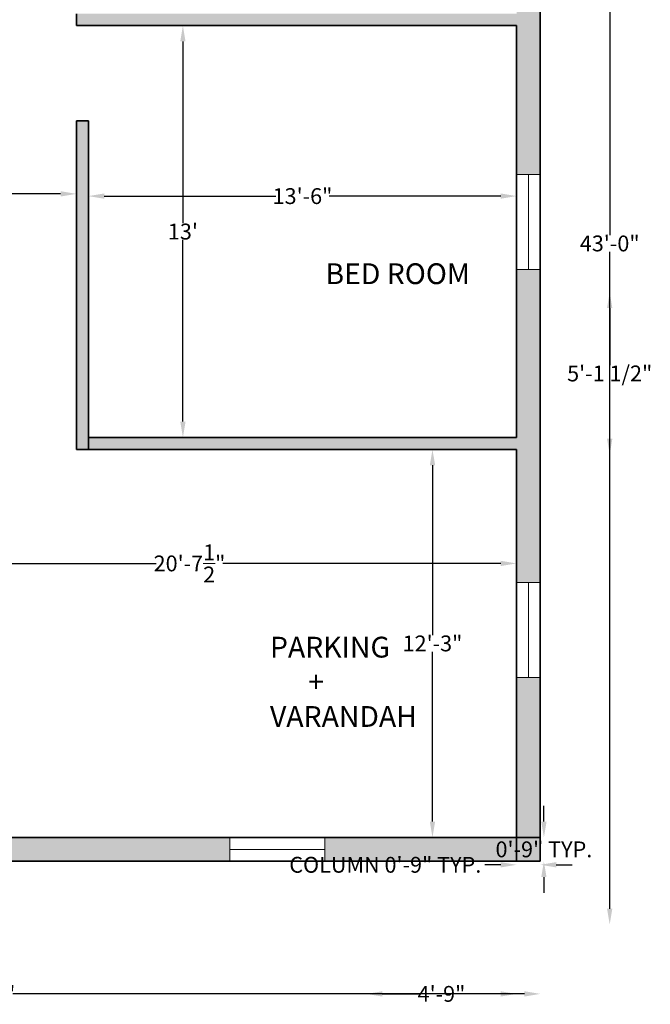
# Model space of a CAD drawing. Units: inches. Extents: x 759 to 1283, y 452 to 1038.
# Tile 2 of 3: x 1044 to 1283, y 457 to 830. Entities that reach past the tile are written whole.
import ezdxf

# ---------------------------------------------------------------- set-up
doc = ezdxf.new("R2010")
doc.units = ezdxf.units.IN
for name, color, linetype, lineweight in [('A-AREA-IDEN', 1, 'Continuous', 25), ('A-COLS', 7, 'Continuous', 35), ('A-COLS-PATT', 7, 'Continuous', 13), ('DIM', 2, 'Continuous', 18), ('WALL', 7, 'Continuous', 35), ('WINDOWS', 4, 'Continuous', 18)]:
    doc.layers.add(name, color=color, linetype=linetype, lineweight=lineweight)
doc.layers.add('A-WALL-PATT', color=67, linetype='Continuous', lineweight=13, true_color=0x727430)
doc.styles.get("Standard").update_dxf_attribs({"font": 'arial.ttf'})
doc.dimstyles.get("Standard").update_dxf_attribs({"dimtxt": 6, "dimasz": 6, "dimexe": 0.18, "dimexo": 0.0625, "dimgap": 0.09, "dimtad": 0, "dimtih": 1, "dimtoh": 1, "dimdec": 4, "dimzin": 0, "dimdsep": 46, "dimlunit": 4, "dimtxsty": 'Standard', "dimcen": 0.09, "dimse1": 1, "dimse2": 1, "dimadec": 0, "dimazin": 0, "dimtfac": 1, "dimtdec": 4, "dimtofl": 0, "dimtmove": 0, "dimatfit": 3, "dimfxl": 1, "dimtolj": 1, "dimtzin": 0, "dimarcsym": 0})

# ---------------------------------------------------------------- blocks, each defined once
blk = doc.blocks.new('*D11')
at = {"layer": 'Defpoints', "color": 0, "transparency": 16777216}
for p in [(1232.47, 666.81), (1200.66, 519.81), (1232.47, 519.81)]:
    blk.add_point(p, dxfattribs=at)
at = {"layer": 'DIM', "color": 0, "lineweight": -2, "transparency": 16777216}
for p, q in [((1200.66, 660.81), (1200.66, 596.46)), ((1200.66, 525.81), (1200.66, 590.15))]:
    blk.add_line(p, q, dxfattribs=at)
at = {"layer": 'DIM', "color": 0, "transparency": 16777216}
for points in [[(1199.66, 660.81), (1201.66, 660.81), (1200.66, 666.81)], [(1199.66, 525.81), (1201.66, 525.81), (1200.66, 519.81)]]:
    blk.add_solid(points, dxfattribs=at)
at = {"layer": 'DIM', "color": 0, "transparency": 16777216, "insert": (1200.66, 593.31), "char_height": 6, "attachment_point": 5}
blk.add_mtext('\\A1;12\'-3"', dxfattribs=at)
blk = doc.blocks.new('*D12')
at = {"layer": 'Defpoints', "color": 0, "transparency": 16777216}
for p in [(1232.47, 623.61), (984.97, 524.08), (1232.47, 524.08)]:
    blk.add_point(p, dxfattribs=at)
at = {"layer": 'DIM', "color": 0, "lineweight": -2, "transparency": 16777216}
for p, q in [((990.97, 623.61), (1096.08, 623.61)), ((1226.47, 623.61), (1121.35, 623.61))]:
    blk.add_line(p, q, dxfattribs=at)
at = {"layer": 'DIM', "color": 0, "transparency": 16777216}
for points in [[(990.97, 624.61), (990.97, 622.61), (984.97, 623.61)], [(1226.47, 624.61), (1226.47, 622.61), (1232.47, 623.61)]]:
    blk.add_solid(points, dxfattribs=at)
at = {"layer": 'DIM', "color": 0, "transparency": 16777216, "insert": (1108.72, 623.61), "char_height": 6, "attachment_point": 5}
blk.add_mtext('\\A1;20\'-7{\\H1x;\\S1/2;}"', dxfattribs=at)
blk = doc.blocks.new('*D13')
at = {"layer": 'Defpoints', "color": 0, "transparency": 16777216}
for p in [(1106.22, 827.31), (1215.11, 827.31), (1215.11, 671.31)]:
    blk.add_point(p, dxfattribs=at)
at = {"layer": 'DIM', "color": 0, "lineweight": -2, "transparency": 16777216}
for p, q in [((1106.22, 821.31), (1106.22, 752.46)), ((1106.22, 677.31), (1106.22, 746.15))]:
    blk.add_line(p, q, dxfattribs=at)
at = {"layer": 'DIM', "color": 0, "transparency": 16777216}
for points in [[(1105.22, 821.31), (1107.22, 821.31), (1106.22, 827.31)], [(1105.22, 677.31), (1107.22, 677.31), (1106.22, 671.31)]]:
    blk.add_solid(points, dxfattribs=at)
at = {"layer": 'DIM', "color": 0, "transparency": 16777216, "insert": (1106.22, 749.31), "char_height": 6, "attachment_point": 5}
blk.add_mtext("\\A1;13'", dxfattribs=at)
blk = doc.blocks.new('*D14')
at = {"layer": 'Defpoints', "color": 0, "transparency": 16777216}
for p in [(1070.47, 775.52), (1232.47, 775.52), (1232.47, 762.74)]:
    blk.add_point(p, dxfattribs=at)
at = {"layer": 'DIM', "color": 0, "lineweight": -2, "transparency": 16777216}
for p, q in [((1076.47, 762.74), (1141.35, 762.74)), ((1226.47, 762.74), (1161.58, 762.74))]:
    blk.add_line(p, q, dxfattribs=at)
at = {"layer": 'DIM', "color": 0, "transparency": 16777216}
for points in [[(1076.47, 763.74), (1076.47, 761.74), (1070.47, 762.74)], [(1226.47, 763.74), (1226.47, 761.74), (1232.47, 762.74)]]:
    blk.add_solid(points, dxfattribs=at)
at = {"layer": 'DIM', "color": 0, "transparency": 16777216, "insert": (1151.47, 762.74), "char_height": 6, "attachment_point": 5}
blk.add_mtext('\\A1;13\'-6"', dxfattribs=at)
blk = doc.blocks.new('*D15')
at = {"layer": 'Defpoints', "color": 0, "transparency": 16777216}
for p in [(1065.97, 763.58), (918.97, 756.35), (1065.97, 756.35)]:
    blk.add_point(p, dxfattribs=at)
at = {"layer": 'DIM', "color": 0, "lineweight": -2, "transparency": 16777216}
for p, q in [((924.97, 763.58), (982.35, 763.58)), ((1059.97, 763.58), (1002.58, 763.58))]:
    blk.add_line(p, q, dxfattribs=at)
at = {"layer": 'DIM', "color": 0, "transparency": 16777216}
for points in [[(924.97, 764.58), (924.97, 762.58), (918.97, 763.58)], [(1059.97, 764.58), (1059.97, 762.58), (1065.97, 763.58)]]:
    blk.add_solid(points, dxfattribs=at)
at = {"layer": 'DIM', "color": 0, "transparency": 16777216, "insert": (992.47, 763.58), "char_height": 6, "attachment_point": 5}
blk.add_mtext('\\A1;12\'-3"', dxfattribs=at)
blk = doc.blocks.new('WIN-36IN')
for p, q in [((0, 0), (0, 9)), ((0, 9), (36, 9)), ((36, 9), (36, 0)), ((0, 4.5), (36, 4.5)), ((36, 0), (0, 0))]:
    blk.add_line(p, q)
blk = doc.blocks.new('COL-9X9IN')
for p, q in [((0, 0), (0, 9)), ((0, 9), (9, 9)), ((9, 9), (9, 0)), ((9, 0), (0, 0))]:
    blk.add_line(p, q)
blk = doc.blocks.new('*D21')
at = {"layer": 'Defpoints', "color": 0, "transparency": 16777216}
for p in [(1232.47, 510.81), (1232.47, 509.46), (1241.47, 510.81)]:
    blk.add_point(p, dxfattribs=at)
at = {"layer": 'DIM', "color": 0, "lineweight": -2, "transparency": 16777216}
for p, q in [((1226.47, 509.46), (1220.47, 509.46)), ((1247.47, 509.46), (1253.47, 509.46))]:
    blk.add_line(p, q, dxfattribs=at)
at = {"layer": 'DIM', "color": 0, "transparency": 16777216}
for points in [[(1226.47, 510.46), (1226.47, 508.46), (1232.47, 509.46)], [(1247.47, 510.46), (1247.47, 508.46), (1241.47, 509.46)]]:
    blk.add_solid(points, dxfattribs=at)
at = {"layer": 'DIM', "color": 0, "transparency": 16777216, "insert": (1182.8, 509.46), "char_height": 6, "attachment_point": 5}
blk.add_mtext('\\A1;COLUMN 0\'-9" TYP.', dxfattribs=at)
blk = doc.blocks.new('*D22')
at = {"layer": 'Defpoints', "color": 0, "transparency": 16777216}
for p in [(1241.47, 519.81), (1241.47, 510.81), (1242.82, 510.81)]:
    blk.add_point(p, dxfattribs=at)
at = {"layer": 'DIM', "color": 0, "lineweight": -2, "transparency": 16777216}
for p, q in [((1242.82, 525.81), (1242.82, 531.81)), ((1242.82, 504.81), (1242.82, 498.81))]:
    blk.add_line(p, q, dxfattribs=at)
at = {"layer": 'DIM', "color": 0, "transparency": 16777216}
for points in [[(1241.82, 525.81), (1243.82, 525.81), (1242.82, 519.81)], [(1241.82, 504.81), (1243.82, 504.81), (1242.82, 510.81)]]:
    blk.add_solid(points, dxfattribs=at)
at = {"layer": 'DIM', "color": 0, "transparency": 16777216, "insert": (1242.82, 515.31), "char_height": 6, "attachment_point": 5}
blk.add_mtext('\\A1;0\'-9" TYP.', dxfattribs=at)
blk = doc.blocks.new('*D23')
at = {"layer": 'Defpoints', "color": 0, "transparency": 16777216}
for p in [(821.47, 510.81), (1241.47, 510.81), (1241.47, 460.56)]:
    blk.add_point(p, dxfattribs=at)
at = {"layer": 'DIM', "color": 0, "lineweight": -2, "transparency": 16777216}
for p, q in [((827.47, 460.56), (1021.07, 460.56)), ((1235.47, 460.56), (1041.86, 460.56))]:
    blk.add_line(p, q, dxfattribs=at)
at = {"layer": 'DIM', "color": 0, "transparency": 16777216}
for points in [[(827.47, 461.56), (827.47, 459.56), (821.47, 460.56)], [(1235.47, 461.56), (1235.47, 459.56), (1241.47, 460.56)]]:
    blk.add_solid(points, dxfattribs=at)
at = {"layer": 'DIM', "color": 0, "transparency": 16777216, "insert": (1031.47, 460.56), "char_height": 6, "attachment_point": 5}
blk.add_mtext('\\A1;35\'-0"', dxfattribs=at)
blk = doc.blocks.new('*D24')
at = {"layer": 'Defpoints', "color": 0, "transparency": 16777216}
for p in [(1070.47, 1002.81), (1267.72, 1002.81), (1032.97, 486.81)]:
    blk.add_point(p, dxfattribs=at)
at = {"layer": 'DIM', "color": 0, "lineweight": -2, "transparency": 16777216}
for p, q in [((1267.72, 996.81), (1267.72, 747.96)), ((1267.72, 492.81), (1267.72, 741.65))]:
    blk.add_line(p, q, dxfattribs=at)
at = {"layer": 'DIM', "color": 0, "transparency": 16777216}
for points in [[(1266.72, 996.81), (1268.72, 996.81), (1267.72, 1002.81)], [(1266.72, 492.81), (1268.72, 492.81), (1267.72, 486.81)]]:
    blk.add_solid(points, dxfattribs=at)
at = {"layer": 'DIM', "color": 0, "transparency": 16777216, "insert": (1267.72, 744.81), "char_height": 6, "attachment_point": 5}
blk.add_mtext('\\A1;43\'-0"', dxfattribs=at)
blk = doc.blocks.new('*D30')
at = {"layer": 'Defpoints', "color": 0, "transparency": 16777216}
for p in [(1175.68, 981.81), (1232.47, 981.81), (1232.47, 460.56)]:
    blk.add_point(p, dxfattribs=at)
at = {"layer": 'DIM', "color": 0, "lineweight": -2, "transparency": 16777216}
for p, q in [((1181.68, 460.56), (1195.89, 460.56)), ((1226.47, 460.56), (1212.26, 460.56))]:
    blk.add_line(p, q, dxfattribs=at)
at = {"layer": 'DIM', "color": 0, "transparency": 16777216}
for points in [[(1181.68, 461.56), (1181.68, 459.56), (1175.68, 460.56)], [(1226.47, 461.56), (1226.47, 459.56), (1232.47, 460.56)]]:
    blk.add_solid(points, dxfattribs=at)
at = {"layer": 'DIM', "color": 0, "transparency": 16777216, "insert": (1204.07, 460.56), "char_height": 6, "attachment_point": 5}
blk.add_mtext('\\A1;4\'-9"', dxfattribs=at)
blk = doc.blocks.new('*D32')
at = {"layer": 'Defpoints', "color": 0, "transparency": 16777216}
for p in [(1232.47, 1029.06), (1159.97, 519.81), (1232.47, 519.81)]:
    blk.add_point(p, dxfattribs=at)
at = {"layer": 'DIM', "color": 0, "lineweight": -2, "transparency": 16777216}
for p, q in [((1165.97, 1029.06), (1181.15, 1029.06)), ((1226.47, 1029.06), (1211.29, 1029.06))]:
    blk.add_line(p, q, dxfattribs=at)
at = {"layer": 'DIM', "color": 0, "transparency": 16777216}
for points in [[(1165.97, 1030.06), (1165.97, 1028.06), (1159.97, 1029.06)], [(1226.47, 1030.06), (1226.47, 1028.06), (1232.47, 1029.06)]]:
    blk.add_solid(points, dxfattribs=at)
at = {"layer": 'DIM', "color": 0, "transparency": 16777216, "insert": (1196.22, 1029.06), "char_height": 6, "attachment_point": 5}
blk.add_mtext('\\A1;6\'-0 1/2"', dxfattribs=at)
blk = doc.blocks.new('*D38')
at = {"layer": 'Defpoints', "color": 0, "transparency": 16777216}
for p in [(795.22, 734.88), (1232.47, 734.88), (1232.47, 671.31)]:
    blk.add_point(p, dxfattribs=at)
at = {"layer": 'DIM', "color": 0, "lineweight": -2, "transparency": 16777216}
for p, q in [((795.22, 728.88), (795.22, 706.29)), ((795.22, 677.31), (795.22, 699.9))]:
    blk.add_line(p, q, dxfattribs=at)
at = {"layer": 'DIM', "color": 0, "transparency": 16777216}
for points in [[(794.22, 728.88), (796.22, 728.88), (795.22, 734.88)], [(794.22, 677.31), (796.22, 677.31), (795.22, 671.31)]]:
    blk.add_solid(points, dxfattribs=at)
at = {"layer": 'DIM', "color": 0, "transparency": 16777216, "insert": (795.22, 703.09), "char_height": 6, "attachment_point": 5}
blk.add_mtext('\\A1;5\'-3 1/2"', dxfattribs=at)
blk = doc.blocks.new('*D39')
at = {"layer": 'Defpoints', "color": 0, "transparency": 16777216}
for p in [(795.22, 580.37), (1232.47, 580.37), (1232.47, 519.81)]:
    blk.add_point(p, dxfattribs=at)
at = {"layer": 'DIM', "color": 0, "lineweight": -2, "transparency": 16777216}
for p, q in [((795.22, 574.37), (795.22, 553.28)), ((795.22, 525.81), (795.22, 546.89))]:
    blk.add_line(p, q, dxfattribs=at)
at = {"layer": 'DIM', "color": 0, "transparency": 16777216}
for points in [[(794.22, 574.37), (796.22, 574.37), (795.22, 580.37)], [(794.22, 525.81), (796.22, 525.81), (795.22, 519.81)]]:
    blk.add_solid(points, dxfattribs=at)
at = {"layer": 'DIM', "color": 0, "transparency": 16777216, "insert": (795.22, 550.09), "char_height": 6, "attachment_point": 5}
blk.add_mtext('\\A1;5\'-0 1/2"', dxfattribs=at)
blk = doc.blocks.new('*D43')
at = {"layer": 'Defpoints', "color": 0, "transparency": 16777216}
for p in [(1070.47, 827.31), (795.22, 791.31), (1070.47, 791.31)]:
    blk.add_point(p, dxfattribs=at)
at = {"layer": 'DIM', "color": 0, "lineweight": -2, "transparency": 16777216}
for p, q in [((795.22, 821.31), (795.22, 812.46)), ((795.22, 797.31), (795.22, 806.15))]:
    blk.add_line(p, q, dxfattribs=at)
at = {"layer": 'DIM', "color": 0, "transparency": 16777216}
for points in [[(794.22, 821.31), (796.22, 821.31), (795.22, 827.31)], [(794.22, 797.31), (796.22, 797.31), (795.22, 791.31)]]:
    blk.add_solid(points, dxfattribs=at)
at = {"layer": 'DIM', "color": 0, "transparency": 16777216, "insert": (795.22, 809.31), "char_height": 6, "attachment_point": 5}
blk.add_mtext('\\A1;3\'-0"', dxfattribs=at)
blk = doc.blocks.new('*D45')
at = {"layer": 'Defpoints', "color": 0, "transparency": 16777216}
for p in [(918.97, 726.32), (980.47, 664.81), (1267.72, 664.81)]:
    blk.add_point(p, dxfattribs=at)
at = {"layer": 'DIM', "color": 0, "lineweight": -2, "transparency": 16777216}
for p, q in [((1267.72, 720.32), (1267.72, 698.76)), ((1267.72, 670.81), (1267.72, 692.37))]:
    blk.add_line(p, q, dxfattribs=at)
at = {"layer": 'DIM', "color": 0, "transparency": 16777216}
for points in [[(1266.72, 720.32), (1268.72, 720.32), (1267.72, 726.32)], [(1266.72, 670.81), (1268.72, 670.81), (1267.72, 664.81)]]:
    blk.add_solid(points, dxfattribs=at)
at = {"layer": 'DIM', "color": 0, "transparency": 16777216, "insert": (1267.72, 695.57), "char_height": 6, "attachment_point": 5}
blk.add_mtext('\\A1;5\'-1 1/2"', dxfattribs=at)

msp = doc.modelspace()

# ---------------------------------------------------------------- hatches: boundary and pattern name
at = {"layer": 'A-COLS-PATT'}
h = msp.add_hatch(color=256, dxfattribs=at)
h.dxf.hatch_style = 1
h.paths.add_polyline_path([(1241.46699, 990.80698), (1232.46699, 990.80698), (1232.46699, 981.80698), (1241.46699, 981.80698)])
h.paths.add_polyline_path([(830.46699, 990.80698), (821.46699, 990.80698), (821.46699, 981.80698), (830.46699, 981.80698)])
h.paths.add_polyline_path([(830.46699, 519.80698), (821.46699, 519.80698), (821.46699, 510.80698), (830.46699, 510.80698)])
h.paths.add_polyline_path([(1241.46699, 519.80698), (1232.46699, 519.80698), (1232.46699, 510.80698), (1241.46699, 510.80698)])
at = {"layer": 'A-WALL-PATT'}
h = msp.add_hatch(color=256, dxfattribs=at)
h.dxf.hatch_style = 1
h.paths.add_polyline_path([(1232.46699, 519.80698), (1159.97269, 519.80698), (1159.97269, 510.80698), (1232.46699, 510.80698)])
h.paths.add_polyline_path([(1241.46699, 580.365), (1232.46699, 580.365), (1232.46699, 519.80698), (1241.46699, 519.80698)])
h.paths.add_polyline_path([(1123.97269, 519.80698), (1032.96699, 519.80698), (1032.96699, 510.80698), (1123.97269, 510.80698)])
h.paths.add_polyline_path([(984.96699, 519.80698), (984.96699, 664.80698), (980.46699, 664.80698), (980.46699, 660.30698), (980.46699, 519.80698), (920.40841, 519.80698), (920.40841, 510.80698), (984.96699, 510.80698)])
h.paths.add_polyline_path([(884.40841, 519.80698), (830.46699, 519.80698), (830.46699, 510.80698), (884.40841, 510.80698)])
h.paths.add_polyline_path([(830.46699, 590.05698), (821.46699, 590.05698), (821.46699, 519.80698), (830.46699, 519.80698)])
h.paths.add_polyline_path([(830.46699, 660.30698), (944.46699, 660.30698), (944.46699, 664.80698), (830.46699, 664.80698), (830.46699, 691.13164), (821.46699, 691.13164), (821.46699, 626.05698), (830.46699, 626.05698)])
h.paths.add_polyline_path([(830.46699, 767.80698), (914.46699, 767.80698), (914.46699, 726.32345), (918.96699, 726.32345), (918.96699, 775.80521), (918.96699, 790.30698), (914.46699, 790.30698), (914.46699, 772.30698), (830.46699, 772.30698), (830.46699, 782.14186), (821.46699, 782.14186), (821.46699, 727.13164), (830.46699, 727.13164)])
h.paths.add_polyline_path([(830.46699, 906.80698), (821.46699, 906.80698), (821.46699, 818.14186), (830.46699, 818.14186), (830.46699, 827.30698), (984.96699, 827.30698), (984.96699, 831.80698), (980.46699, 831.80698), (830.46699, 831.80698)])
h.paths.add_polyline_path([(830.46699, 981.80698), (821.46699, 981.80698), (821.46699, 942.80698), (830.46699, 942.80698)])
h.paths.add_polyline_path([(884.40841, 990.80698), (830.46699, 990.80698), (830.46699, 981.80698), (884.40841, 981.80698)])
h.paths.add_polyline_path([(984.96699, 998.30698), (1065.96699, 998.30698), (1065.96699, 981.80698), (1065.96699, 867.80698), (1070.46699, 867.80698), (1070.46699, 981.80698), (1139.68016, 981.80698), (1139.68016, 990.80698), (1070.46699, 990.80698), (1070.46699, 1002.80698), (980.46699, 1002.80698), (980.46699, 990.80698), (920.40841, 990.80698), (920.40841, 981.80698), (980.46699, 981.80698), (980.46699, 867.80698), (984.96699, 867.80698), (984.96699, 981.80698)])
h.paths.add_polyline_path([(1232.46699, 990.80698), (1175.68016, 990.80698), (1175.68016, 981.80698), (1232.46699, 981.80698)])
h.paths.add_polyline_path([(1241.46699, 981.80698), (1232.46699, 981.80698), (1232.46699, 947.03418), (1241.46699, 947.03418)])
h.paths.add_polyline_path([(1241.46699, 911.03418), (1232.46699, 911.03418), (1232.46699, 831.80698), (1070.46699, 831.80698), (1065.96699, 831.80698), (1065.96699, 827.30698), (1070.46699, 827.30698), (1232.46699, 827.30698), (1232.46699, 770.87725), (1241.46699, 770.87725)])
h.paths.add_polyline_path([(1241.46699, 734.87725), (1232.46699, 734.87725), (1232.46699, 671.30698), (1070.46699, 671.30698), (1070.46699, 666.80698), (1232.46699, 666.80698), (1232.46699, 616.365), (1241.46699, 616.365)])
h.paths.add_polyline_path([(1070.46699, 791.30698), (1065.96699, 791.30698), (1065.96699, 666.80698), (1070.46699, 666.80698)])

# ---------------------------------------------------------------- linework, layer by layer
at = {"layer": 'WALL'}
for p, q in [((1241.46699, 990.80698), (1241.46699, 510.80698)), ((1065.96699, 831.80698), (1065.96699, 827.30698)), ((1065.96699, 827.30698), (1070.46699, 827.30698)), ((1070.46699, 827.30698), (1232.46699, 827.30698)), ((1232.46699, 827.30698), (1232.46699, 671.30698)), ((1065.96699, 791.30698), (1065.96699, 666.80698)), ((1070.46699, 791.30698), (1065.96699, 791.30698)), ((1070.46699, 791.30698), (1070.46699, 666.80698)), ((1070.46699, 791.30698), (1070.46699, 791.30698)), ((1070.46699, 671.30698), (1232.46699, 671.30698)), ((1065.96699, 666.80698), (1232.46699, 666.80698)), ((1232.46699, 666.80698), (1232.46699, 519.80698)), ((1032.96699, 519.80698), (1232.46699, 519.80698)), ((821.46699, 510.80698), (1241.46699, 510.80698))]:
    msp.add_line(p, q, dxfattribs=at)

# ---------------------------------------------------------------- block references
at = {"layer": 'A-COLS', "rotation": 180}
msp.add_blockref('COL-9X9IN', (1241.46697, 519.80696), dxfattribs=at)
at = {"layer": 'WINDOWS', "rotation": 270.0000000000004}
for p in [(1232.46701, 770.87766), (1232.46701, 616.36541)]:
    msp.add_blockref('WIN-36IN', p, dxfattribs=at)
at = {"layer": 'WINDOWS'}
msp.add_blockref('WIN-36IN', (1123.97228, 510.807), dxfattribs=at)

# ---------------------------------------------------------------- texts
at = {"layer": 'A-AREA-IDEN', "char_height": 7.875, "attachment_point": 1}
for s, insert in [('BED ROOM', (1160.16986, 737.27594)), ('PARKING \\P      +\\PVARANDAH', (1139.1768, 595.83406))]:
    msp.add_mtext_dynamic_manual_height_columns(s, width=120.4934303, gutter_width=39.375, heights=[0], dxfattribs=dict(at, insert=insert))

# ---------------------------------------------------------------- dimensions: what is measured, and where the dimension line sits
at = {"layer": 'DIM'}
for base, p1, p2, override, picture, middle in [((1232.46699, 1029.05698), (1159.97269, 519.80698), (1232.46699, 519.80698), {"dimdec": 1, "dimlfac": 1, "dimrnd": 0, "dimzin": 1, "dimdsep": 46, "dimlunit": 4, "dimfrac": 2}, '*D32', (1196.21984, 1029.05698)), ((1232.46699, 460.55698), (1175.68016, 981.80698), (1232.46699, 981.80698), {"dimdec": 1, "dimlfac": 1, "dimrnd": 0, "dimzin": 1, "dimdsep": 46, "dimlunit": 4, "dimfrac": 2}, '*D30', (1204.07357, 460.55698)), ((1232.46699, 762.7372), (1070.46699, 775.5204), (1232.46699, 775.5204), {"dimclrd": 0, "dimclre": 0, "dimclrt": 0}, '*D14', (1151.46699, 762.7372)), ((1065.96699, 763.57787), (918.96699, 756.34782), (1065.96699, 756.34782), {"dimclrd": 0, "dimclre": 0, "dimclrt": 0}, '*D15', (992.46699, 763.57787)), ((1232.46699, 623.61456), (984.96699, 524.07962), (1232.46699, 524.07962), {"dimclrd": 0, "dimclre": 0, "dimclrt": 0}, '*D12', (1108.71699, 623.61456)), ((1241.46699, 460.55698), (821.46699, 510.80698), (1241.46699, 510.80698), {"dimdec": 1, "dimlfac": 1, "dimrnd": 0, "dimzin": 1, "dimdsep": 46, "dimlunit": 4, "dimfrac": 2}, '*D23', (1031.46699, 460.55698))]:
    dim = msp.add_linear_dim(base=base, p1=p1, p2=p2, dimstyle='Standard', override=override, dxfattribs=at)
    dim.commit()
    dim.dimension.update_dxf_attribs({"geometry": picture, "text_midpoint": middle})
for base, p1, p2, override, picture, middle in [((1267.71699, 1002.80698), (1032.96699, 486.80698), (1070.46699, 1002.80698), {"dimdec": 1, "dimlfac": 1, "dimrnd": 0, "dimzin": 1, "dimdsep": 46, "dimlunit": 4, "dimfrac": 2}, '*D24', (1267.71699, 744.80698)), ((795.21699, 791.30698), (1070.46699, 827.30698), (1070.46699, 791.30698), {"dimdec": 1, "dimlfac": 1, "dimrnd": 0, "dimzin": 1, "dimdsep": 46, "dimlunit": 4, "dimfrac": 2}, '*D43', (795.21699, 809.30698)), ((1106.22122, 827.30698), (1215.10726, 671.30698), (1215.10726, 827.30698), {"dimclrd": 0, "dimclre": 0, "dimclrt": 0}, '*D13', (1106.22122, 749.30698)), ((795.21699, 734.87725), (1232.46699, 671.30698), (1232.46699, 734.87725), {"dimdec": 1, "dimlfac": 1, "dimrnd": 0, "dimzin": 1, "dimdsep": 46, "dimlunit": 4, "dimfrac": 2}, '*D38', (795.21699, 703.09212)), ((1267.71699, 664.80698), (918.96699, 726.32345), (980.46699, 664.80698), {"dimdec": 1, "dimlfac": 1, "dimrnd": 0, "dimzin": 1, "dimdsep": 46, "dimlunit": 4, "dimfrac": 2}, '*D45', (1267.71699, 695.56521)), ((1200.66012, 519.80698), (1232.46699, 666.80698), (1232.46699, 519.80698), {"dimclrd": 0, "dimclre": 0, "dimclrt": 0}, '*D11', (1200.66012, 593.30698)), ((795.21699, 580.365), (1232.46699, 519.80698), (1232.46699, 580.365), {"dimdec": 1, "dimlfac": 1, "dimrnd": 0, "dimzin": 1, "dimdsep": 46, "dimlunit": 4, "dimfrac": 2}, '*D39', (795.21699, 550.08599))]:
    dim = msp.add_linear_dim(base=base, p1=p1, p2=p2, angle=90, dimstyle='Standard', override=override, dxfattribs=at)
    dim.commit()
    dim.dimension.update_dxf_attribs({"geometry": picture, "text_midpoint": middle})
for base, p1, p2, angle, text, picture, middle in [((1242.81699, 510.80698), (1241.46699, 519.80698), (1241.46699, 510.80698), 270, '<> TYP.', '*D22', (1242.81699, 515.30698)), ((1232.46699, 509.45698), (1241.46699, 510.80698), (1232.46699, 510.80698), 180, 'COLUMN <> TYP.', '*D21', (1182.79922, 509.45698))]:
    dim = msp.add_linear_dim(base=base, p1=p1, p2=p2, angle=angle, text=text, dimstyle='Standard', override={"dimdec": 1, "dimlfac": 1, "dimrnd": 0, "dimzin": 1, "dimdsep": 46, "dimlunit": 4, "dimfrac": 2}, dxfattribs=at)
    dim.commit()
    dim.dimension.update_dxf_attribs({"geometry": picture, "text_midpoint": middle})

doc.saveas('drawing.dxf')
